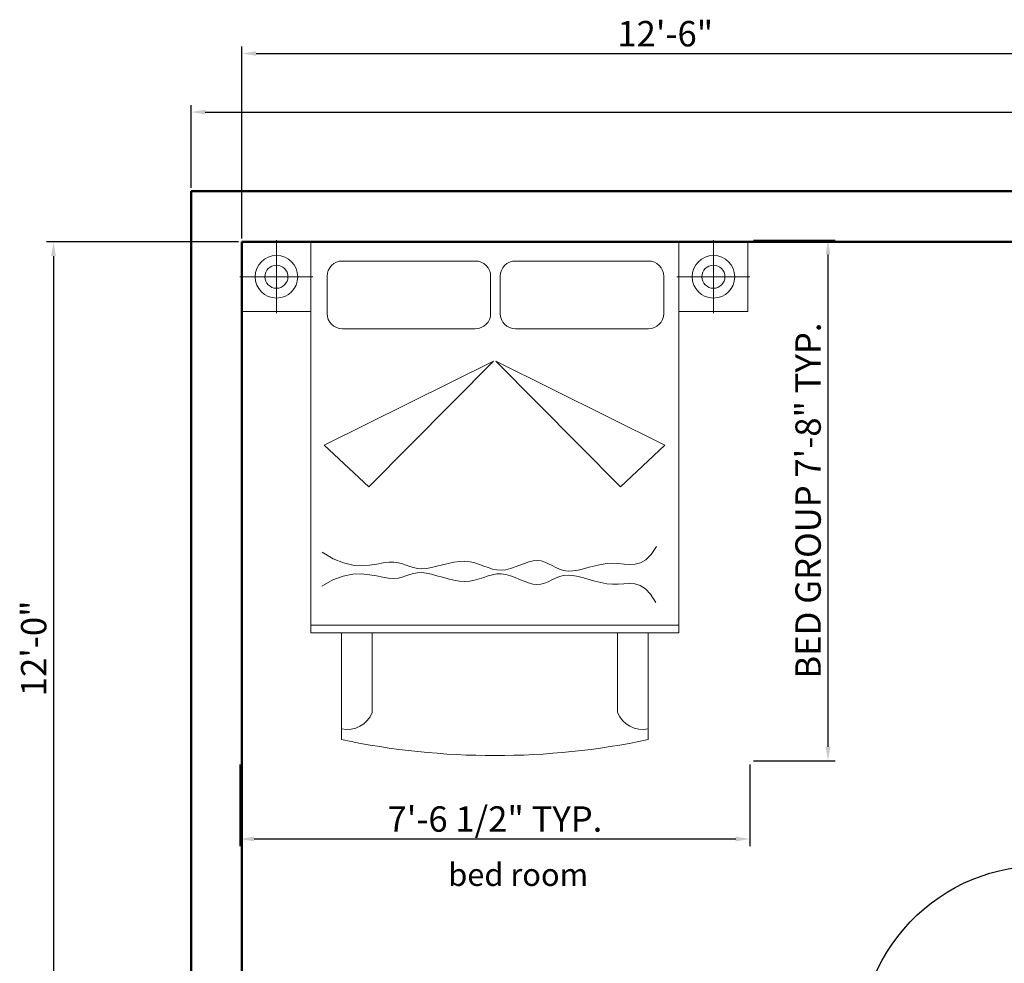
# Model space of a CAD drawing. Units: inches. Extents: x 1253 to 1645, y 2180 to 2698.
# Tile 3 of 5: x 1257 to 1431, y 2531 to 2698. Entities that reach past the tile are written whole.
import ezdxf

# ---------------------------------------------------------------- set-up
doc = ezdxf.new("R2010")
doc.units = ezdxf.units.IN
for name, color, linetype, lineweight in [('A-ANNO-DIMS', 2, 'Continuous', 18), ('A-AREA-IDEN', 7, 'Continuous', 25), ('A-DOOR', 4, 'Continuous', 25), ('A-FURN', 8, 'Continuous', 18), ('wall', 7, 'Continuous', 50)]:
    doc.layers.add(name, color=color, linetype=linetype, lineweight=lineweight)
doc.styles.get("Standard").update_dxf_attribs({"font": 'arial.ttf'})
doc.dimstyles.new('ISO-25', dxfattribs={"dimtxt": 4.5, "dimasz": 2.5, "dimexe": 1.25, "dimexo": 0.625, "dimtad": 1, "dimdec": 1, "dimlunit": 3, "dimtxsty": 'Standard', "dimcen": 4.5, "dimadec": 0, "dimazin": 0, "dimtfac": 1, "dimtdec": 1, "dimtmove": 0, "dimatfit": 3, "dimfxl": 1, "dimarcsym": 0})

# ---------------------------------------------------------------- blocks, each defined once
blk = doc.blocks.new('A$C4F543DC7')
for p, q in [((0.0134, 3.35, -0.1688), (3.3134, 3.35, -0.1688)), ((0.4634, 3.35, -0.1688), (0.0134, 3.35, -0.1688)), ((0.0134, 2.896, -0.1688), (0.0134, 3.35, -0.1688)), ((0.0134, 3.35, -0.1688), (0.0134, 2.896, -0.1688)), ((0.2381, 3.1233, -0.4388), (0.2381, 3.3614, -0.4388)), ((0.4634, 3.35, -0.1688), (0.4634, 0.8, -0.1688)), ((2.8634, 3.35, -0.1688), (0.4634, 3.35, -0.1688)), ((0.4634, 2.896, -0.1688), (0.4634, 3.35, -0.1688)), ((2.8634, 0.8, -0.1688), (2.8634, 3.35, -0.1688)), ((2.8634, 3.35, -0.1688), (3.3134, 3.35, -0.1688)), ((2.8634, 2.896, -0.1688), (2.8634, 3.35, -0.1688)), ((3.0888, 3.1233, -0.4388), (3.0888, 3.3614, -0.4388)), ((3.3134, 3.35, -0.1688), (3.3134, 2.896, -0.1688)), ((3.3134, 3.35, -0.1688), (3.3134, 2.896, -0.1688)), ((1.5354, 3.226, -0.1688), (0.6684, 3.226, -0.1688)), ((2.6644, 3.226, -0.1688), (1.7974, 3.226, -0.1688)), ((0.2381, 3.1233, -0.4388), (0, 3.1233, -0.4388)), ((0.2381, 3.1233, -0.4388), (0.4762, 3.1233, -0.4388)), ((0.2381, 3.1233, -0.4388), (0.2381, 2.8852, -0.4388)), ((0.5684, 3.126, -0.1688), (0.5684, 2.884, -0.1688)), ((1.6354, 2.884, -0.1688), (1.6354, 3.126, -0.1688)), ((1.6974, 3.126, -0.1688), (1.6974, 2.884, -0.1688)), ((2.7644, 2.884, -0.1688), (2.7644, 3.126, -0.1688)), ((3.0888, 3.1233, -0.4388), (2.8507, 3.1233, -0.4388)), ((3.0888, 3.1233, -0.4388), (3.0888, 2.8852, -0.4388)), ((3.0888, 3.1233, -0.4388), (3.3269, 3.1233, -0.4388)), ((0.4634, 2.896, -0.1688), (0.0134, 2.896, -0.1688)), ((0.0134, 2.896, -0.1688), (0.4634, 2.896, -0.1688)), ((0.4634, 0.8, -0.1688), (0.4634, 2.896, -0.1688)), ((2.8634, 2.896, -0.1688), (2.8634, 0.8, -0.1688)), ((3.3134, 2.896, -0.1688), (2.8634, 2.896, -0.1688)), ((3.3134, 2.896, -0.1688), (2.8634, 2.896, -0.1688)), ((0.6684, 2.784, -0.1688), (1.5354, 2.784, -0.1688)), ((1.7974, 2.784, -0.1688), (2.6644, 2.784, -0.1688)), ((1.6534, 2.573, -0.1688), (0.5504, 2.025, -0.1688)), ((0.8414, 1.752, -0.1688), (1.6534, 2.573, -0.1688)), ((2.4814, 1.752, -0.1688), (1.6694, 2.573, -0.1688)), ((1.6694, 2.573, -0.1688), (2.7724, 2.025, -0.1688)), ((0.5504, 2.025, -0.1688), (0.8414, 1.752, -0.1688)), ((2.7724, 2.025, -0.1688), (2.4814, 1.752, -0.1688)), ((2.683, 1.312, -0.1688), (2.7182, 1.3641, -0.1688)), ((0.5369, 1.3267, -0.1688), (0.6088, 1.2835, -0.1688)), ((2.6479, 1.2774, -0.1688), (2.683, 1.312, -0.1688)), ((0.6088, 1.2835, -0.1688), (0.6756, 1.2566, -0.1688)), ((0.6756, 1.2566, -0.1688), (0.7373, 1.2428, -0.1688)), ((0.7373, 1.2428, -0.1688), (0.794, 1.239, -0.1688)), ((0.794, 1.239, -0.1688), (0.8457, 1.242, -0.1688)), ((0.8457, 1.242, -0.1688), (0.8925, 1.2489, -0.1688)), ((0.8925, 1.2489, -0.1688), (0.9345, 1.2564, -0.1688)), ((0.9345, 1.2564, -0.1688), (0.9718, 1.2615, -0.1688)), ((0.9718, 1.2615, -0.1688), (1.0044, 1.2617, -0.1688)), ((1.0044, 1.2617, -0.1688), (1.0334, 1.2578, -0.1688)), ((1.0334, 1.2578, -0.1688), (1.0597, 1.2509, -0.1688)), ((1.0597, 1.2509, -0.1688), (1.0842, 1.2424, -0.1688)), ((1.0842, 1.2424, -0.1688), (1.1081, 1.2336, -0.1688)), ((1.1081, 1.2336, -0.1688), (1.1322, 1.2257, -0.1688)), ((1.1322, 1.2257, -0.1688), (1.1577, 1.2201, -0.1688)), ((1.1855, 1.218, -0.1688), (1.2163, 1.2204, -0.1688)), ((1.2163, 1.2204, -0.1688), (1.2498, 1.2264, -0.1688)), ((1.2498, 1.2264, -0.1688), (1.2852, 1.2347, -0.1688)), ((1.2852, 1.2347, -0.1688), (1.3218, 1.2441, -0.1688)), ((1.3218, 1.2441, -0.1688), (1.3591, 1.2533, -0.1688)), ((1.3591, 1.2533, -0.1688), (1.3963, 1.2612, -0.1688)), ((1.3963, 1.2612, -0.1688), (1.4328, 1.2664, -0.1688)), ((1.4328, 1.2664, -0.1688), (1.4679, 1.2677, -0.1688)), ((1.4679, 1.2677, -0.1688), (1.501, 1.2643, -0.1688)), ((1.501, 1.2643, -0.1688), (1.5324, 1.257, -0.1688)), ((1.5324, 1.257, -0.1688), (1.5624, 1.2473, -0.1688)), ((1.5624, 1.2473, -0.1688), (1.5915, 1.2365, -0.1688)), ((1.5915, 1.2365, -0.1688), (1.6199, 1.2259, -0.1688)), ((1.6199, 1.2259, -0.1688), (1.6481, 1.2169, -0.1688)), ((1.7651, 1.2199, -0.1688), (1.7955, 1.2301, -0.1688)), ((1.7955, 1.2301, -0.1688), (1.8258, 1.2417, -0.1688)), ((1.8258, 1.2417, -0.1688), (1.8557, 1.2531, -0.1688)), ((1.8557, 1.2531, -0.1688), (1.8849, 1.263, -0.1688)), ((1.8849, 1.263, -0.1688), (1.913, 1.2698, -0.1688)), ((1.913, 1.2698, -0.1688), (1.9397, 1.2722, -0.1688)), ((1.9397, 1.2722, -0.1688), (1.9649, 1.2692, -0.1688)), ((1.9649, 1.2692, -0.1688), (1.989, 1.2617, -0.1688)), ((1.989, 1.2617, -0.1688), (2.0124, 1.2512, -0.1688)), ((2.0124, 1.2512, -0.1688), (2.0359, 1.2391, -0.1688)), ((2.0359, 1.2391, -0.1688), (2.0599, 1.2269, -0.1688)), ((2.0599, 1.2269, -0.1688), (2.0849, 1.216, -0.1688)), ((2.242, 1.2182, -0.1688), (2.2791, 1.2279, -0.1688)), ((2.2791, 1.2279, -0.1688), (2.3173, 1.2378, -0.1688)), ((2.3173, 1.2378, -0.1688), (2.3558, 1.2465, -0.1688)), ((2.3558, 1.2465, -0.1688), (2.3944, 1.2527, -0.1688)), ((2.3944, 1.2527, -0.1688), (2.4325, 1.255, -0.1688)), ((2.4325, 1.255, -0.1688), (2.4698, 1.2529, -0.1688)), ((2.4698, 1.2529, -0.1688), (2.5064, 1.2488, -0.1688)), ((2.5064, 1.2488, -0.1688), (2.5423, 1.2459, -0.1688)), ((2.5423, 1.2459, -0.1688), (2.5777, 1.2476, -0.1688)), ((2.5777, 1.2476, -0.1688), (2.6129, 1.257, -0.1688)), ((2.6129, 1.257, -0.1688), (2.6479, 1.2774, -0.1688)), ((0.6067, 1.1458, -0.1688), (0.6743, 1.1706, -0.1688)), ((0.6743, 1.1706, -0.1688), (0.7364, 1.1825, -0.1688)), ((0.7364, 1.1825, -0.1688), (0.7931, 1.1846, -0.1688)), ((0.7931, 1.1846, -0.1688), (0.8447, 1.1799, -0.1688)), ((0.8447, 1.1799, -0.1688), (0.8913, 1.1716, -0.1688)), ((0.8913, 1.1716, -0.1688), (0.9331, 1.1628, -0.1688)), ((0.9331, 1.1628, -0.1688), (0.9701, 1.1565, -0.1688)), ((0.9701, 1.1565, -0.1688), (1.0027, 1.1552, -0.1688)), ((1.0027, 1.1552, -0.1688), (1.0318, 1.1582, -0.1688)), ((1.0318, 1.1582, -0.1688), (1.0583, 1.1642, -0.1688)), ((1.0583, 1.1642, -0.1688), (1.0831, 1.172, -0.1688)), ((1.0831, 1.172, -0.1688), (1.1072, 1.18, -0.1688)), ((1.1072, 1.18, -0.1688), (1.1316, 1.1872, -0.1688)), ((1.1316, 1.1872, -0.1688), (1.1573, 1.192, -0.1688)), ((1.1573, 1.192, -0.1688), (1.1851, 1.1932, -0.1688)), ((1.1577, 1.2201, -0.1688), (1.1855, 1.218, -0.1688)), ((1.1851, 1.1932, -0.1688), (1.2158, 1.1898, -0.1688)), ((1.2158, 1.1898, -0.1688), (1.2491, 1.1828, -0.1688)), ((1.2491, 1.1828, -0.1688), (1.2842, 1.1734, -0.1688)), ((1.2842, 1.1734, -0.1688), (1.3206, 1.1629, -0.1688)), ((1.3206, 1.1629, -0.1688), (1.3575, 1.1524, -0.1688)), ((1.5609, 1.152, -0.1688), (1.5903, 1.1619, -0.1688)), ((1.5903, 1.1619, -0.1688), (1.6191, 1.1716, -0.1688)), ((1.6191, 1.1716, -0.1688), (1.6475, 1.1797, -0.1688)), ((1.6475, 1.1797, -0.1688), (1.676, 1.1849, -0.1688)), ((1.6481, 1.2169, -0.1688), (1.6765, 1.2108, -0.1688)), ((1.676, 1.1849, -0.1688), (1.7049, 1.1858, -0.1688)), ((1.6765, 1.2108, -0.1688), (1.7053, 1.209, -0.1688)), ((1.7049, 1.1858, -0.1688), (1.7344, 1.1816, -0.1688)), ((1.7053, 1.209, -0.1688), (1.7349, 1.2124, -0.1688)), ((1.7344, 1.1816, -0.1688), (1.7643, 1.1731, -0.1688)), ((1.7349, 1.2124, -0.1688), (1.7651, 1.2199, -0.1688)), ((1.7643, 1.1731, -0.1688), (1.7944, 1.1619, -0.1688)), ((1.7944, 1.1619, -0.1688), (1.8244, 1.1494, -0.1688)), ((2.0344, 1.1454, -0.1688), (2.0588, 1.1568, -0.1688)), ((2.0588, 1.1568, -0.1688), (2.0842, 1.167, -0.1688)), ((2.0842, 1.167, -0.1688), (2.1112, 1.1743, -0.1688)), ((2.0849, 1.216, -0.1688), (2.1117, 1.2077, -0.1688)), ((2.1112, 1.1743, -0.1688), (2.1403, 1.1775, -0.1688)), ((2.1117, 1.2077, -0.1688), (2.1407, 1.2037, -0.1688)), ((2.1403, 1.1775, -0.1688), (2.1718, 1.1755, -0.1688)), ((2.1407, 1.2037, -0.1688), (2.1723, 1.2047, -0.1688)), ((2.1718, 1.1755, -0.1688), (2.2056, 1.1691, -0.1688)), ((2.1723, 1.2047, -0.1688), (2.2062, 1.21, -0.1688)), ((2.2056, 1.1691, -0.1688), (2.2411, 1.1598, -0.1688)), ((2.2062, 1.21, -0.1688), (2.242, 1.2182, -0.1688)), ((2.2411, 1.1598, -0.1688), (2.2779, 1.1489, -0.1688)), ((0.5334, 1.105, -0.1688), (0.6067, 1.1458, -0.1688)), ((1.3575, 1.1524, -0.1688), (1.3945, 1.1434, -0.1688)), ((1.3945, 1.1434, -0.1688), (1.4308, 1.1371, -0.1688)), ((1.4308, 1.1371, -0.1688), (1.4658, 1.1347, -0.1688)), ((1.4658, 1.1347, -0.1688), (1.499, 1.137, -0.1688)), ((1.499, 1.137, -0.1688), (1.5306, 1.1433, -0.1688)), ((1.5306, 1.1433, -0.1688), (1.5609, 1.152, -0.1688)), ((1.8244, 1.1494, -0.1688), (1.8539, 1.137, -0.1688)), ((1.8539, 1.137, -0.1688), (1.8827, 1.1263, -0.1688)), ((1.8827, 1.1263, -0.1688), (1.9106, 1.1186, -0.1688)), ((1.9106, 1.1186, -0.1688), (1.9373, 1.1153, -0.1688)), ((1.9373, 1.1153, -0.1688), (1.9625, 1.1176, -0.1688)), ((1.9625, 1.1176, -0.1688), (1.9868, 1.1243, -0.1688)), ((1.9868, 1.1243, -0.1688), (2.0106, 1.134, -0.1688)), ((2.0106, 1.134, -0.1688), (2.0344, 1.1454, -0.1688)), ((2.2779, 1.1489, -0.1688), (2.3157, 1.1379, -0.1688)), ((2.3157, 1.1379, -0.1688), (2.354, 1.1279, -0.1688)), ((2.354, 1.1279, -0.1688), (2.3923, 1.1205, -0.1688)), ((2.3923, 1.1205, -0.1688), (2.4304, 1.117, -0.1688)), ((2.4304, 1.117, -0.1688), (2.4677, 1.118, -0.1688)), ((2.4677, 1.118, -0.1688), (2.5043, 1.1209, -0.1688)), ((2.5043, 1.1209, -0.1688), (2.5403, 1.1226, -0.1688)), ((2.5403, 1.1226, -0.1688), (2.5757, 1.1199, -0.1688)), ((2.5757, 1.1199, -0.1688), (2.6106, 1.1094, -0.1688)), ((2.6106, 1.1094, -0.1688), (2.645, 1.0879, -0.1688)), ((2.645, 1.0879, -0.1688), (2.6789, 1.0522, -0.1688)), ((2.6789, 1.0522, -0.1688), (2.7124, 0.999, -0.1688)), ((0.4634, 0.85, -0.1688), (2.8634, 0.85, -0.1688)), ((0.4634, 0.8, -0.1688), (2.8634, 0.8, -0.1688)), ((0.6634, 0.8, -0.1688), (0.4634, 0.8, -0.1688)), ((0.6634, 0.8, -0.1688), (2.6634, 0.8, -0.1688)), ((0.6634, 0.104, -0.1688), (0.6634, 0.8, -0.1688)), ((0.6634, 0.104, -0.1688), (0.6634, 0.8, -0.1688)), ((0.8634, 0.281, -0.1688), (0.8634, 0.8, -0.1688)), ((2.4634, 0.8, -0.1688), (2.4634, 0.281, -0.1688)), ((2.8634, 0.8, -0.1688), (2.6634, 0.8, -0.1688)), ((2.6634, 0.8, -0.1688), (2.6634, 0.104, -0.1688)), ((2.6634, 0.8, -0.1688), (2.6634, 0.104, -0.1688))]:
    blk.add_line(p, q)
for centre, radius in [((0.2381, 3.1233, -0.4388), 0.139), ((3.0888, 3.1233, -0.4388), 0.139), ((0.2381, 3.1233, -0.4388), 0.075), ((3.0888, 3.1233, -0.4388), 0.075)]:
    blk.add_circle(centre, radius)
for centre, radius, start, end in [((0.6684, 3.126, -0.1688), 0.1, 90, 180), ((1.5354, 3.126, -0.1688), 0.1, 0, 90), ((1.7974, 3.126, -0.1688), 0.1, 90, 180), ((2.6644, 3.126, -0.1688), 0.1, 0, 90), ((0.6684, 2.884, -0.1688), 0.1, 180, 270), ((1.5354, 2.884, -0.1688), 0.1, 270, 0), ((1.7974, 2.884, -0.1688), 0.1, 180, 270), ((2.6644, 2.884, -0.1688), 0.1, 270, 0), ((0.6994, 0.3472, -0.1688), 0.1769, 258.2616, 338.03196), ((2.6275, 0.3472, -0.1688), 0.1769, 201.96804, 281.7384), ((1.6634, 4.8597, -0.1688), 4.8597, 258.12517, 281.87483), ((1.6634, 4.8597, -0.1688), 4.8597, 258.12517, 281.87483)]:
    blk.add_arc(centre, radius, start, end)
blk = doc.blocks.new('*D13')
at = {"layer": 'A-ANNO-DIMS', "color": 0, "lineweight": -2, "transparency": 16777216}
for p, q in [((1286.94, 2667.97), (1286.94, 2682.62)), ((1616.94, 2667.97), (1616.94, 2682.62)), ((1289.44, 2681.37), (1614.44, 2681.37))]:
    blk.add_line(p, q, dxfattribs=at)
at = {"layer": 'A-ANNO-DIMS', "color": 0, "transparency": 16777216}
for points in [[(1289.44, 2681.79), (1289.44, 2680.95), (1286.94, 2681.37)], [(1614.44, 2681.79), (1614.44, 2680.95), (1616.94, 2681.37)]]:
    blk.add_solid(points, dxfattribs=at)
at = {"layer": 'Defpoints', "color": 0, "transparency": 16777216}
for p in [(1616.94, 2681.37), (1286.94, 2667.35), (1616.94, 2667.35)]:
    blk.add_point(p, dxfattribs=at)
at = {"layer": 'A-ANNO-DIMS', "color": 0, "transparency": 16777216, "insert": (1451.94, 2684.29), "char_height": 4.5, "attachment_point": 5}
blk.add_mtext('27\'-6"', dxfattribs=at)
blk = doc.blocks.new('DOOR-SWING-36IN')
for p, q in [((1.5, 1.5), (1.5, 37.5)), ((3, 1.5), (3, 37.5)), ((0, 3), (0, 0)), ((1.5, 3), (0, 3)), ((1.5, 1.5), (1.5, 3)), ((34.5, 1.5), (34.5, 3)), ((34.5, 3), (36, 3)), ((36, 3), (36, 0)), ((3, 1.5), (1.5, 1.5)), ((3, 0), (3, 1.5)), ((33, 0), (33, 1.5)), ((33, 1.5), (34.5, 1.5)), ((0, 0), (3, 0)), ((36, 0), (33, 0))]:
    blk.add_line(p, q)
blk.add_arc((2.25, 5.18), 32.32, 356.1244, 91.3295)
blk = doc.blocks.new('*D18')
at = {"layer": 'A-ANNO-DIMS', "color": 0, "lineweight": -2, "transparency": 16777216}
for p, q in [((1386.57, 2658.66), (1401.03, 2658.66)), ((1399.78, 2568.91), (1399.78, 2656.16)), ((1386.57, 2566.41), (1401.03, 2566.41))]:
    blk.add_line(p, q, dxfattribs=at)
at = {"layer": 'A-ANNO-DIMS', "color": 0, "transparency": 16777216}
for points in [[(1399.37, 2656.16), (1400.2, 2656.16), (1399.78, 2658.66)], [(1399.37, 2568.91), (1400.2, 2568.91), (1399.78, 2566.41)]]:
    blk.add_solid(points, dxfattribs=at)
at = {"layer": 'Defpoints', "color": 0, "transparency": 16777216}
for p in [(1385.94, 2658.66), (1399.78, 2658.66), (1385.94, 2566.41)]:
    blk.add_point(p, dxfattribs=at)
at = {"layer": 'A-ANNO-DIMS', "color": 0, "transparency": 16777216, "insert": (1396.83, 2612.53), "char_height": 4.5, "attachment_point": 5, "rotation": 90}
blk.add_mtext('BED GROUP 7\'-8" TYP.', dxfattribs=at)
blk = doc.blocks.new('*D19')
at = {"layer": 'A-ANNO-DIMS', "color": 0, "lineweight": -2, "transparency": 16777216}
for p, q in [((1295.58, 2565.78), (1295.58, 2551.32)), ((1385.94, 2565.78), (1385.94, 2551.32)), ((1298.08, 2552.57), (1383.44, 2552.57))]:
    blk.add_line(p, q, dxfattribs=at)
at = {"layer": 'A-ANNO-DIMS', "color": 0, "transparency": 16777216}
for points in [[(1298.08, 2552.99), (1298.08, 2552.15), (1295.58, 2552.57)], [(1383.44, 2552.99), (1383.44, 2552.15), (1385.94, 2552.57)]]:
    blk.add_solid(points, dxfattribs=at)
at = {"layer": 'Defpoints', "color": 0, "transparency": 16777216}
for p in [(1295.58, 2566.41), (1385.94, 2566.41), (1385.94, 2552.57)]:
    blk.add_point(p, dxfattribs=at)
at = {"layer": 'A-ANNO-DIMS', "color": 0, "transparency": 16777216, "insert": (1340.76, 2555.52), "char_height": 4.5, "attachment_point": 5}
blk.add_mtext('7\'-6 1/2" TYP.', dxfattribs=at)
blk = doc.blocks.new('*D28')
at = {"layer": 'A-ANNO-DIMS', "color": 0, "lineweight": -2, "transparency": 16777216}
for p, q in [((1295.94, 2658.97), (1295.94, 2693)), ((1445.94, 2658.97), (1445.94, 2693)), ((1298.44, 2691.75), (1443.44, 2691.75))]:
    blk.add_line(p, q, dxfattribs=at)
at = {"layer": 'A-ANNO-DIMS', "color": 0, "transparency": 16777216}
for points in [[(1298.44, 2692.16), (1298.44, 2691.33), (1295.94, 2691.75)], [(1443.44, 2692.16), (1443.44, 2691.33), (1445.94, 2691.75)]]:
    blk.add_solid(points, dxfattribs=at)
at = {"layer": 'Defpoints', "color": 0, "transparency": 16777216}
for p in [(1445.94, 2691.75), (1295.94, 2658.35), (1445.94, 2658.35)]:
    blk.add_point(p, dxfattribs=at)
at = {"layer": 'A-ANNO-DIMS', "color": 0, "transparency": 16777216, "insert": (1370.94, 2694.67), "char_height": 4.5, "attachment_point": 5}
blk.add_mtext('12\'-6"', dxfattribs=at)
blk = doc.blocks.new('*D30')
at = {"layer": 'A-ANNO-DIMS', "color": 0, "lineweight": -2, "transparency": 16777216}
for p, q in [((1295.32, 2658.35), (1261.29, 2658.35)), ((1262.54, 2655.85), (1262.54, 2516.85)), ((1295.32, 2514.35), (1261.29, 2514.35))]:
    blk.add_line(p, q, dxfattribs=at)
at = {"layer": 'A-ANNO-DIMS', "color": 0, "transparency": 16777216}
for points in [[(1262.12, 2655.85), (1262.96, 2655.85), (1262.54, 2658.35)], [(1262.12, 2516.85), (1262.96, 2516.85), (1262.54, 2514.35)]]:
    blk.add_solid(points, dxfattribs=at)
at = {"layer": 'Defpoints', "color": 0, "transparency": 16777216}
for p in [(1295.94, 2658.35), (1262.54, 2514.35), (1295.94, 2514.35)]:
    blk.add_point(p, dxfattribs=at)
at = {"layer": 'A-ANNO-DIMS', "color": 0, "transparency": 16777216, "insert": (1259.62, 2586.35), "char_height": 4.5, "attachment_point": 5, "rotation": 90}
blk.add_mtext('12\'-0"', dxfattribs=at)

msp = doc.modelspace()

# ---------------------------------------------------------------- linework, layer by layer
at = {"layer": 'wall'}
for p, q in [((1616.94, 2667.35), (1286.94, 2667.35)), ((1286.94, 2667.35), (1286.94, 2205.35)), ((1607.94, 2658.35), (1295.94, 2658.35)), ((1295.94, 2658.35), (1295.94, 2214.35))]:
    msp.add_line(p, q, dxfattribs=at)

# ---------------------------------------------------------------- block references
at = {"layer": 'A-DOOR', "extrusion": (0, 0, -1), "zscale": -1}
msp.add_blockref('DOOR-SWING-36IN', (-1439.94, 2510.35), dxfattribs=at)
at = {"layer": 'A-FURN', "xscale": 27.16316877811709, "yscale": 27.16316877811709, "zscale": 27.16316877811709}
msp.add_blockref('A$C4F543DC7', (1295.58, 2567.35, 4.58), dxfattribs=at)

# ---------------------------------------------------------------- texts
at = {"layer": 'A-AREA-IDEN', "insert": (1332.49, 2548.25), "char_height": 4, "attachment_point": 1}
msp.add_mtext_dynamic_manual_height_columns('bed room', width=71.3777, gutter_width=12.5, heights=[0], dxfattribs=at)

# ---------------------------------------------------------------- dimensions: what is measured, and where the dimension line sits
at = {"layer": 'A-ANNO-DIMS'}
for base, p1, p2, override, picture, middle in [((1445.94, 2691.75), (1295.94, 2658.35), (1445.94, 2658.35), {"dimdec": 1, "dimlfac": 1, "dimrnd": 0, "dimzin": 1, "dimdsep": 46, "dimlunit": 4, "dimfrac": 2}, '*D28', (1370.94, 2694.67)), ((1616.94, 2681.37), (1286.94, 2667.35), (1616.94, 2667.35), {"dimclrd": 0, "dimclre": 0, "dimclrt": 0}, '*D13', (1451.94, 2684.29))]:
    dim = msp.add_linear_dim(base=base, p1=p1, p2=p2, dimstyle='ISO-25', override=override, dxfattribs=at)
    dim.commit()
    dim.dimension.update_dxf_attribs({"geometry": picture, "text_midpoint": middle})
dim = msp.add_linear_dim(base=(1262.54, 2514.35), p1=(1295.94, 2658.35), p2=(1295.94, 2514.35), angle=90, dimstyle='ISO-25', override={"dimdec": 1, "dimlfac": 1, "dimrnd": 0, "dimzin": 1, "dimdsep": 46, "dimlunit": 4, "dimfrac": 2}, dxfattribs=at)
dim.commit()
dim.dimension.update_dxf_attribs({"geometry": '*D30', "text_midpoint": (1259.62, 2586.35)})
dim = msp.add_linear_dim(base=(1399.7819, 2658.6555), p1=(1385.9448, 2566.4082), p2=(1385.9448, 2658.6555), angle=90, text='BED GROUP <> TYP.', dimstyle='ISO-25', override={"dimdec": 1, "dimlfac": 1, "dimrnd": 0, "dimzin": 1, "dimdsep": 46, "dimlunit": 4, "dimfrac": 2}, dxfattribs=at)
dim.commit()
dim.dimension.update_dxf_attribs({"geometry": '*D18', "text_midpoint": (1396.8287, 2612.5319)})
dim = msp.add_linear_dim(base=(1385.94, 2552.57), p1=(1295.58, 2566.41), p2=(1385.94, 2566.41), text='<> TYP.', dimstyle='ISO-25', override={"dimdec": 1, "dimlfac": 1, "dimrnd": 0, "dimzin": 1, "dimdsep": 46, "dimlunit": 4, "dimfrac": 2}, dxfattribs=at)
dim.commit()
dim.dimension.update_dxf_attribs({"geometry": '*D19', "text_midpoint": (1340.76, 2555.52)})

doc.saveas('drawing.dxf')
